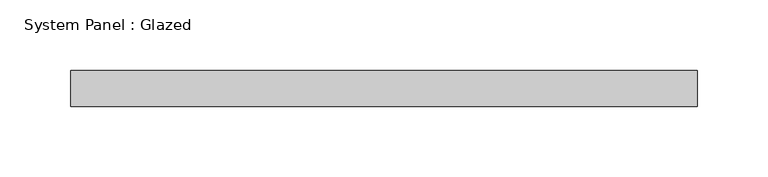
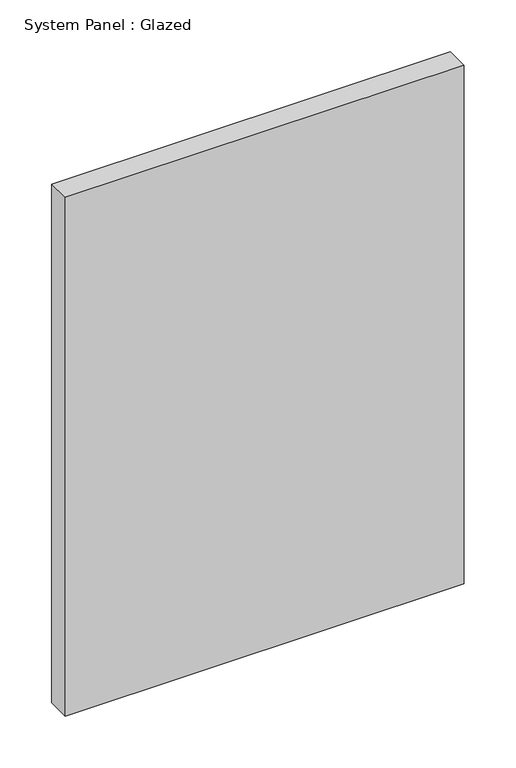
"""IFC4 building model written with IfcOpenShell, lengths in millimetres: plate geometry, System Panel : Glazed."""

from ifc_helpers import new_model, si_unit, origin, origin_with_axes, place, context, project, spatial, polyline, outline, extrude, source, transform, mapped, element, save


def system_panel_glazed_d508e32f(model_context):
    return source(origin(), model_context, "Body", "SweptSolid", [
        extrude(outline(polyline([(221.7349132, 19.05), (-221.7349132, 19.05), (-221.7349132, 44.45), (221.7349132, 44.45), (221.7349132, 19.05)])), origin_with_axes(), (0.0, 0.0, 1.0), 609.6),
    ])


if __name__ == "__main__":
    model = new_model("IFC4")
    model_context = context("Model", 3, world=origin())
    ifc_project = project(units=[si_unit("LENGTHUNIT", "METRE", prefix="MILLI")], contexts=[model_context])
    site = spatial("IfcSite", under=ifc_project)
    building = spatial("IfcBuilding", under=site)
    placement = place(None, origin())
    system_panel_glazed_shape = system_panel_glazed_d508e32f(model_context)
    element("IfcPlate", 1, ObjectType="System Panel : Glazed", at=placement, inside=building, context=model_context, shape_type="MappedRepresentation", body=[
        mapped(system_panel_glazed_shape, transform((0.0, 0.0, 0.0), x_axis=(1.0, 0.0, 0.0), y_axis=(0.0, 1.0, 0.0), z_axis=(0.0, 0.0, 1.0))),
    ])
    save(model, "model.ifc")

# Revit data of these elements
# Type "System Panel : Glazed"
#   Construction Type Id = "GSP4R"
#   Analytic Construction = "1/8 in Pilkington single glazing"
#   Visual Light Transmittance = 0.9
#   Solar Heat Gain Coefficient = 0.86
#   Heat Transfer Coefficient (U) = 1.18115 BTU/(h·ft²·°F)
# Element 1 (IfcPlate, "System Panel : Glazed")
#   Materials on its faces: "Glass"
# Materials
#   "Glass": class "Glass", colour RGB 0 128 192, transparency 0.75, Description = "Soda Lime Glass", Cost = 0
